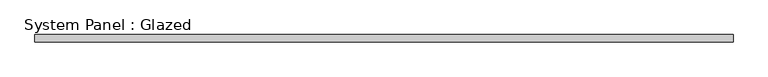
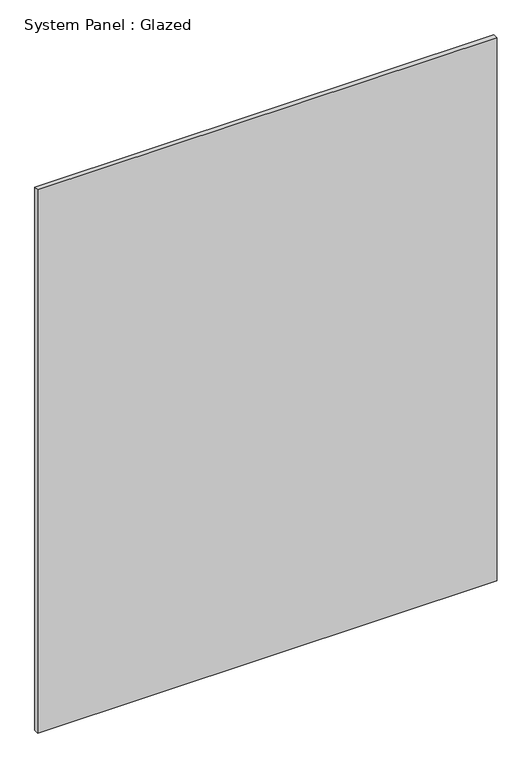
"""IFC4 building model written with IfcOpenShell, lengths in millimetres: plate geometry, System Panel : Glazed."""

from ifc_helpers import new_model, si_unit, origin, origin_with_axes, place, context, project, spatial, polyline, outline, extrude, source, transform, mapped, element, save


def system_panel_glazed_c60cfc80(model_context):
    return source(origin(), model_context, "Body", "SweptSolid", [
        extrude(outline(polyline([(1219.2, 19.05), (-1219.2, 19.05), (-1219.2, 44.45), (1219.2, 44.45), (1219.2, 19.05)])), origin_with_axes(), (0.0, 0.0, 1.0), 3048.0),
    ])


if __name__ == "__main__":
    model = new_model("IFC4")
    model_context = context("Model", 3, world=origin())
    ifc_project = project(units=[si_unit("LENGTHUNIT", "METRE", prefix="MILLI")], contexts=[model_context])
    site = spatial("IfcSite", under=ifc_project)
    building = spatial("IfcBuilding", under=site)
    placement = place(None, origin())
    system_panel_glazed_shape = system_panel_glazed_c60cfc80(model_context)
    element("IfcPlate", 1, ObjectType="System Panel : Glazed", at=placement, inside=building, context=model_context, shape_type="MappedRepresentation", body=[
        mapped(system_panel_glazed_shape, transform((0.0, 0.0, 0.0), x_axis=(1.0, 0.0, 0.0), y_axis=(0.0, 1.0, 0.0), z_axis=(0.0, 0.0, 1.0))),
    ])
    save(model, "model.ifc")

# Revit data of these elements
# Type "System Panel : Glazed"
#   Construction Type Id = "GSP4R"
#   Analytic Construction = "1/8 in Pilkington single glazing"
#   Visual Light Transmittance = 0.9
#   Solar Heat Gain Coefficient = 0.86
#   Heat Transfer Coefficient (U) = 1.18115 BTU/(h·ft²·°F)
#   Define Thermal Properties by = 1
# Element 1 (IfcPlate, "System Panel : Glazed")
#   Materials on its faces: "Glass"
# Materials
#   "Glass": class "Glass", colour RGB 0 128 192, transparency 0.75, Description = "Soda Lime Glass", Cost = 0
